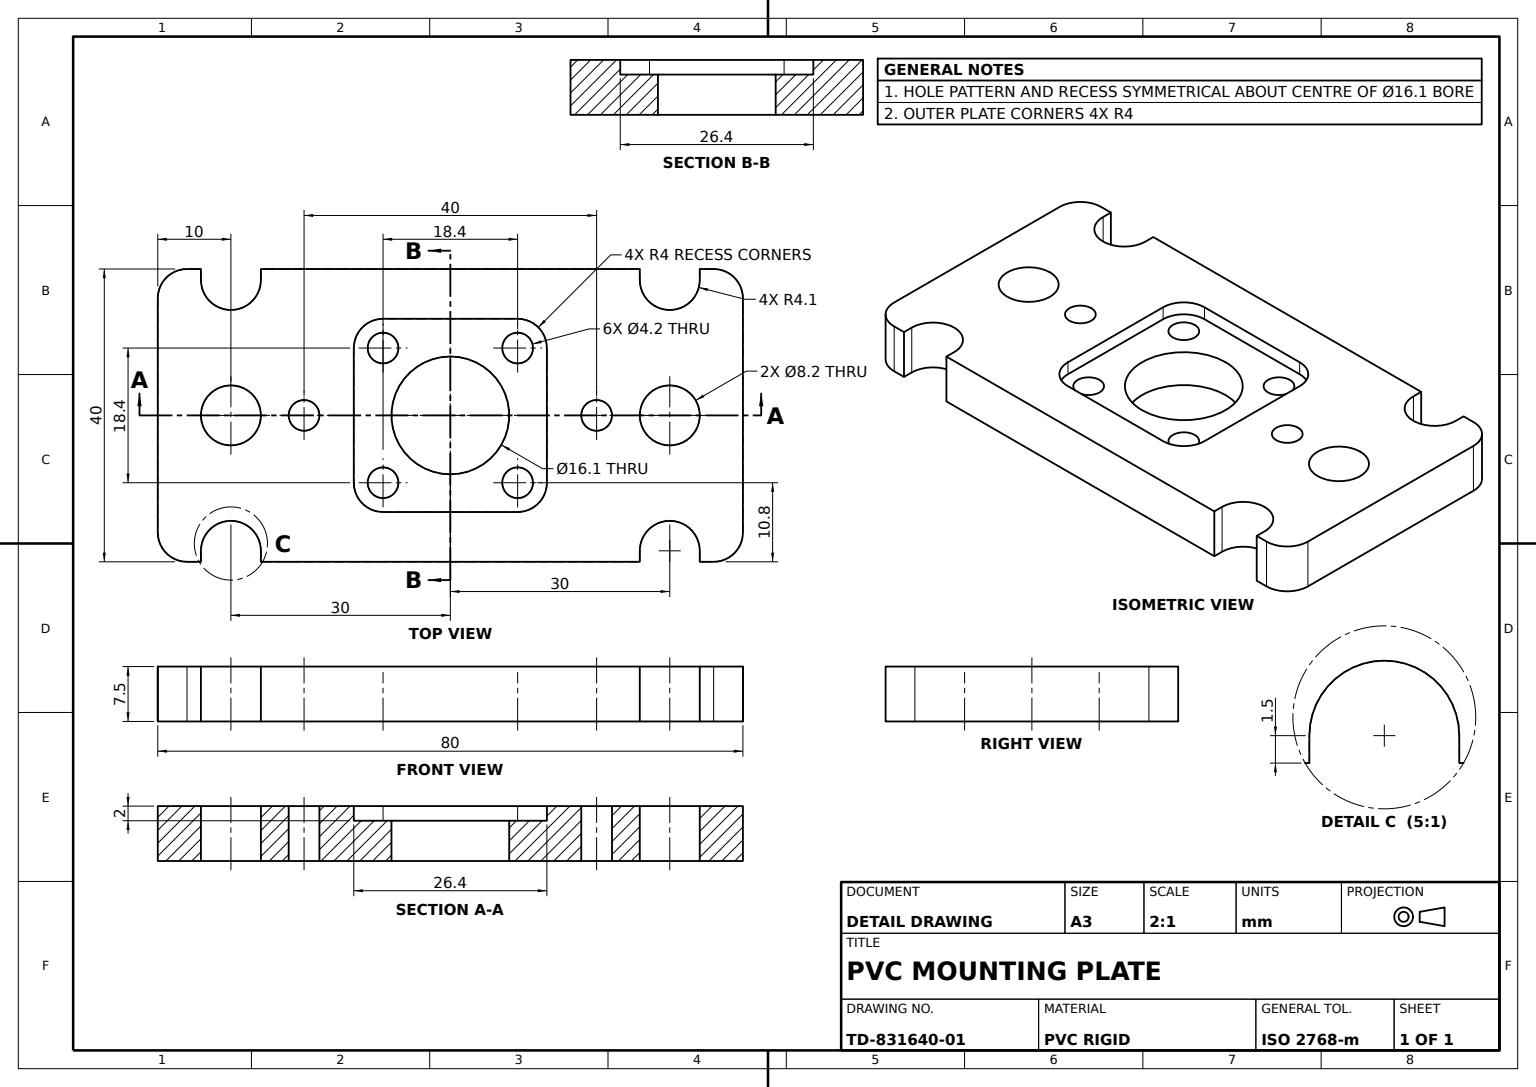
SolidWorks part; units mm, degrees
material "PVC Rigid"
ref_plane "Front Plane" through (0, 0, 0) normal (0, 0, 1) x (1, 0, 0)
ref_plane "Top Plane" through (0, 0, 0) normal (0, 1, 0) x (1, 0, 0)
ref_plane "Right Plane" through (0, 0, 0) normal (1, 0, 0) x (0, 0, -1)
sketch "Base Plate Profile Sketch" plane through (0, 0, 0) normal (0, 1, 0) x (1, 0, 0)
  line L0 (-34.1, 20) -> (-34.1, 18.5)
  line L1 (-36, -20) -> (-34.1, -20)
  line L2 (-40, -16) -> (-40, 16)
  line L3 (-36, 20) -> (-34.1, 20)
  line L4 (40, -16) -> (40, 16)
  line L5 (-40, -20) -> (40, 20) construction
  line L6 (-40, 20) -> (40, -20) construction
  line L7 (-25.9, 18.5) -> (-25.9, 20)
  line L8 (-25.9, 20) -> (25.9, 20)
  line L9 (25.9, 20) -> (25.9, 18.5)
  line L10 (34.1, 18.5) -> (34.1, 20)
  line L11 (34.1, 20) -> (36, 20)
  line L12 (0, 0) -> (-74.6298, 0) construction
  line L13 (34.1, -18.5) -> (34.1, -20)
  line L14 (25.9, -20) -> (25.9, -18.5)
  line L15 (-34.1, -20) -> (-34.1, -18.5)
  line L16 (-25.9, -18.5) -> (-25.9, -20)
  line L17 (34.1, -20) -> (36, -20)
  line L18 (-25.9, -20) -> (25.9, -20)
  line L19 (0, 0) -> (0, -42.2906) construction
  arc A0 (40, 16) -> (36, 20) centre (36, 16) ccw
  arc A1 (40, -16) -> (36, -20) centre (36, -16) cw
  arc A2 (-40, -16) -> (-36, -20) centre (-36, -16) ccw
  arc A3 (-40, 16) -> (-36, 20) centre (-36, 16) cw
  arc A4 (-34.1, 18.5) -> (-25.9, 18.5) centre (-30, 18.5) ccw
  arc A5 (25.9, 18.5) -> (34.1, 18.5) centre (30, 18.5) ccw
  arc A6 (25.9, -18.5) -> (34.1, -18.5) centre (30, -18.5) cw
  arc A7 (-34.1, -18.5) -> (-25.9, -18.5) centre (-30, -18.5) cw
  circle A8 centre (-30, 0) radius 4.1
  circle A9 centre (30, 0) radius 4.1
  circle A10 centre (-20, 0) radius 2.1
  circle A11 centre (20, 0) radius 2.1
  point P0 (0, 0)
  dimension "D3" = 4
  dimension "D5" = 4.1
  dimension "D9" = 8.2
  dimension "D10" = 4.2
  dimension "D1" = 80
  dimension "D2" = 40
  dimension "D4" = 1.5
  dimension "D6" = 30
  dimension "D7" = 2
  dimension "D8" = 10
  dimension "D11" = 10
extrude "Base Plate 7.5mm" add sketch "Base Plate Profile Sketch" along normal blind 7.5
sketch "Connector Recess Sketch" plane through (0, 7.5, 0) normal (0, 1, 0) x (1, 0, 0)
  line L1 (-9.2, -13.2) -> (9.2, -13.2)
  line L2 (-13.2, -9.2) -> (-13.2, 9.2)
  line L3 (-9.2, 13.2) -> (9.2, 13.2)
  line L4 (13.2, -9.2) -> (13.2, 9.2)
  line L5 (-13.2, -13.2) -> (13.2, 13.2) construction
  line L6 (-13.2, 13.2) -> (13.2, -13.2) construction
  arc A0 (-13.2, -9.2) -> (-9.2, -13.2) centre (-9.2, -9.2) ccw
  arc A1 (9.2, -13.2) -> (13.2, -9.2) centre (9.2, -9.2) ccw
  arc A2 (13.2, 9.2) -> (9.2, 13.2) centre (9.2, 9.2) ccw
  arc A3 (-9.2, 13.2) -> (-13.2, 9.2) centre (-9.2, 9.2) ccw
  point P0 (0, 0)
  dimension "D2" = 4
  dimension "D1" = 26.4
extrude "Connector Recess 26.4mm x 2mm" cut sketch "Connector Recess Sketch" against normal blind 2
sketch "Connector Bore and Screw Holes Sketch" plane through (0, 5.5, 0) normal (0, 1, 0) x (1, 0, 0)
  line L0 (0, 0) -> (0, 26.7839) construction
  line L1 (0, 0) -> (-56.8026, 0) construction
  circle A0 centre (0, 0) radius 8.05
  circle A1 centre (-9.2, 9.2) radius 2.1
  arc A2 (-9.2, 13.2) -> (-13.2, 9.2) centre (-9.2, 9.2) ccw construction
  circle A3 centre (-9.2, -9.2) radius 2.1
  circle A4 centre (9.2, -9.2) radius 2.1
  circle A5 centre (9.2, 9.2) radius 2.1
  dimension "D1" = 16.1
  dimension "D2" = 4.2
extrude "Connector Bore and Screw Holes" cut sketch "Connector Bore and Screw Holes Sketch" against normal up to next
